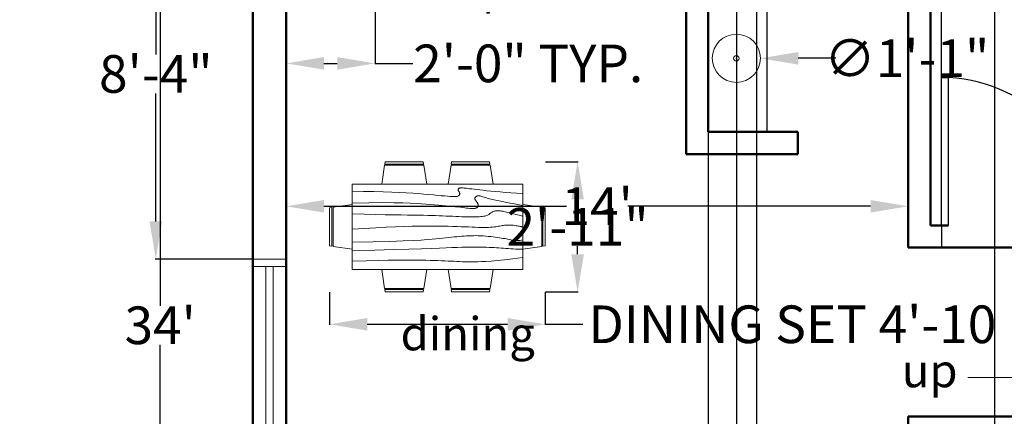
# Model space of a CAD drawing. Units: inches. Extents: x 20 to 3619, y 7 to 1288.
# Tile 2 of 4: x 3080 to 3346, y 967 to 1074. Entities that reach past the tile are written whole.
import ezdxf

# ---------------------------------------------------------------- set-up
doc = ezdxf.new("R2010")
doc.units = ezdxf.units.IN
doc.header["$MEASUREMENT"] = 0
for name, color, linetype, lineweight in [('A-ANNO-DIMS', 2, 'Continuous', 18), ('A-ANNO-SYMB', 7, 'Continuous', 18), ('A-ANNO-TEXT', 7, 'Continuous', 18), ('A-AREA-IDEN', 7, 'Continuous', 25), ('A-DOOR', 3, 'Continuous', 25), ('A-FLOR-CASE', 9, 'Continuous', 25), ('A-FLOR-FIXT', 9, 'Continuous', 18), ('A-FURN', 8, 'Continuous', 18), ('A-GLAZ', 4, 'Continuous', 18), ('A-WALL', 7, 'Continuous', 50)]:
    doc.layers.add(name, color=color, linetype=linetype, lineweight=lineweight)
doc.styles.get("Standard").update_dxf_attribs({"font": 'arial.ttf'})
doc.dimstyles.get("Standard").update_dxf_attribs({"dimtxt": 10.18, "dimasz": 10.18, "dimexe": 0.18, "dimexo": 0.0625, "dimgap": 0.09, "dimtad": 0, "dimtih": 1, "dimtoh": 1, "dimdec": 0, "dimzin": 0, "dimdsep": 46, "dimlunit": 3, "dimtxsty": 'Standard', "dimcen": 0.09, "dimadec": 0, "dimazin": 0, "dimtfac": 1, "dimtdec": 0, "dimtofl": 0, "dimtmove": 0, "dimatfit": 3, "dimfxl": 1, "dimtolj": 1, "dimtzin": 0, "dimarcsym": 0})

# ---------------------------------------------------------------- blocks, each defined once
blk = doc.blocks.new('*D4')
at = {"layer": 'A-ANNO-DIMS', "color": 0, "lineweight": -2, "transparency": 16777216}
for p, q in [((3142.66, 1195.69), (3117.53, 1195.69)), ((3117.71, 1185.51), (3117.71, 996.98)), ((3117.71, 797.87), (3117.71, 986.4)), ((3142.66, 787.69), (3117.53, 787.69))]:
    blk.add_line(p, q, dxfattribs=at)
at = {"layer": 'A-ANNO-DIMS', "color": 0, "transparency": 16777216}
for points in [[(3116.01, 1185.51), (3119.4, 1185.51), (3117.71, 1195.69)], [(3116.01, 797.87), (3119.4, 797.87), (3117.71, 787.69)]]:
    blk.add_solid(points, dxfattribs=at)
at = {"layer": 'Defpoints', "color": 0, "transparency": 16777216}
for p in [(3117.71, 1195.69), (3142.72, 1195.69), (3142.72, 787.69)]:
    blk.add_point(p, dxfattribs=at)
at = {"layer": 'A-ANNO-DIMS', "color": 0, "transparency": 16777216, "insert": (3117.71, 991.69), "char_height": 10.18, "attachment_point": 5}
blk.add_mtext("\\A1;34'", dxfattribs=at)
blk = doc.blocks.new('*U2')
for p, q in [((0, 0), (0, -6)), ((40, 0), (40, -6))]:
    blk.add_line(p, q)
blk.add_lwpolyline([(0, 0), (0, 40), (1.75, 40), (1.75, 0)], close=True)
blk.add_arc((0, 0), 40, 0, 90)
blk = doc.blocks.new('Dining Set - 36 x 72 in.')
for p, q in [((-22.2343, 26.00059), (-23.4847, 17.99762)), ((-22.2304, 26), (-5.7608, 26)), ((-22, 27.5), (-22.1562, 26.50042)), ((-5.8416, 26.5), (-22.1534, 26.5)), ((-22, 27.5), (-6, 27.5)), ((-5.8437, 26.49966), (-6, 27.5)), ((-4.5152, 17.99762), (-5.7655, 25.99926)), ((5.7657, 26.00059), (4.5153, 17.99762)), ((5.7696, 26), (22.2392, 26)), ((6, 27.5), (5.8438, 26.50042)), ((22.1584, 26.5), (5.8466, 26.5)), ((6, 27.5), (22, 27.5)), ((22.1563, 26.49966), (22, 27.5)), ((23.4848, 17.99762), (22.2345, 25.99926)), ((36, 18), (-36, 18)), ((-36, 18), (-36, -18)), ((36, -18), (36, 18)), ((-44.0006, 8.23428), (-35.9976, 9.48474)), ((44.0006, 8.23428), (35.9976, 9.48474)), ((-45.5, 8), (-44.5004, 8.15617)), ((-45.5, 8), (-45.5, -8)), ((-44.5, -8.15843), (-44.5, 8.15338)), ((-44, 8.23041), (-44, -8.23915)), ((44, 8.23041), (44, -8.23915)), ((44.5, -8.15843), (44.5, 8.15338)), ((45.5, 8), (44.5005, 8.15617)), ((45.5, 8), (45.5, -8)), ((-44.4997, -8.15631), (-45.5, -8)), ((-35.9976, -9.48476), (-43.9993, -8.2345)), ((35.9976, -9.48476), (43.9993, -8.2345)), ((44.4997, -8.15631), (45.5, -8)), ((-36, -18), (36, -18)), ((-22.2343, -26.0006), (-23.4847, -17.99762)), ((-4.5152, -17.99762), (-5.7655, -25.99928)), ((5.7657, -26.0006), (4.5153, -17.99762)), ((23.4848, -17.99762), (22.2345, -25.99928)), ((-22.2304, -26), (-5.7608, -26)), ((-22, -27.5), (-22.1562, -26.50044)), ((-5.8416, -26.5), (-22.1534, -26.5)), ((-22, -27.5), (-6, -27.5)), ((-5.8437, -26.49967), (-6, -27.5)), ((5.7696, -26), (22.2392, -26)), ((6, -27.5), (5.8438, -26.50044)), ((22.1584, -26.5), (5.8466, -26.5)), ((6, -27.5), (22, -27.5)), ((22.1563, -26.49967), (22, -27.5))]:
    blk.add_line(p, q)
for points in [[(-36, 15), (-31.1772, 14.97754), (-26.8079, 14.91406), (-22.8538, 14.81543), (-19.276, 14.6875), (-16.0362, 14.53613), (-13.0957, 14.36718), (-10.4159, 14.18652), (-7.9583, 14), (-5.6904, 13.81315), (-3.6035, 13.63021), (-1.6954, 13.45508), (0.0365, 13.29166), (1.5945, 13.14388), (2.9811, 13.01562), (4.1988, 12.9108), (5.25, 12.83333), (6.1393, 12.78613), (6.8802, 12.76823), (7.4883, 12.77767), (7.9792, 12.8125), (8.3685, 12.87077), (8.6719, 12.95052), (8.9049, 13.0498), (9.0833, 13.16666), (9.2205, 13.29899), (9.3216, 13.44401), (9.3895, 13.59879), (9.4271, 13.76041), (9.4373, 13.92594), (9.4232, 14.09245), (9.3875, 14.257), (9.3333, 14.41666), (9.2638, 14.56917), (9.1836, 14.71484), (9.0975, 14.85465), (9.0104, 14.98958), (8.9272, 15.1206), (8.8529, 15.2487), (8.7922, 15.37483), (8.75, 15.5), (8.7305, 15.62467), (8.7344, 15.74739), (8.7617, 15.86621), (8.8125, 15.97916), (8.8867, 16.08431), (8.9844, 16.17968), (9.1055, 16.26334), (9.25, 16.33333), (9.4189, 16.38802), (9.6172, 16.42708), (9.8506, 16.45052), (10.125, 16.45833), (10.4463, 16.45052), (10.8203, 16.42708), (11.2529, 16.38802), (11.75, 16.33333), (12.3184, 16.26318), (12.9694, 16.17838), (13.7151, 16.07991), (14.5677, 15.96875), (15.5395, 15.84586), (16.6426, 15.71224), (17.8893, 15.56884), (19.2917, 15.41666), (20.859, 15.25667), (22.5879, 15.08984), (24.4721, 14.91715), (26.5052, 14.73958), (28.6809, 14.5581), (30.9929, 14.3737), (33.4347, 14.18733), (36, 14)], [(-36, 10), (-28.9766, 10.14274), (-23.1725, 10.20442), (-18.4241, 10.19775), (-14.5677, 10.13541), (-11.4399, 10.03011), (-8.877, 9.89453), (-6.7154, 9.74137), (-4.7917, 9.58333), (-2.9698, 9.43082), (-1.2246, 9.28515), (0.4415, 9.14534), (2.026, 9.01041), (3.5266, 8.87939), (4.9408, 8.7513), (6.266, 8.62516), (7.5, 8.5), (8.6411, 8.37549), (9.6914, 8.2539), (10.6538, 8.13818), (11.5312, 8.03125), (12.3267, 7.93603), (13.043, 7.85547), (13.6831, 7.79248), (14.25, 7.75), (14.7471, 7.7303), (15.1797, 7.73307), (15.5537, 7.75732), (15.875, 7.80208), (16.1494, 7.86637), (16.3828, 7.94922), (16.5811, 8.04964), (16.75, 8.16666), (16.8944, 8.29915), (17.0143, 8.44531), (17.1089, 8.60319), (17.1771, 8.77083), (17.218, 8.94629), (17.2305, 9.1276), (17.2137, 9.31282), (17.1667, 9.5), (17.0895, 9.6875), (16.987, 9.875), (16.8649, 10.0625), (16.7292, 10.25), (16.5856, 10.4375), (16.4401, 10.625), (16.2985, 10.8125), (16.1667, 11), (16.05, 11.18733), (15.9518, 11.3737), (15.8752, 11.5581), (15.8229, 11.73958), (15.798, 11.91715), (15.8034, 12.08984), (15.842, 12.25667), (15.9167, 12.41666), (16.0295, 12.56836), (16.1784, 12.70833), (16.3605, 12.83268), (16.5729, 12.9375), (16.8127, 13.01888), (17.0768, 13.07291), (17.3625, 13.0957), (17.6667, 13.08333), (17.9894, 13.03312), (18.3418, 12.94726), (18.7382, 12.82918), (19.1927, 12.68229), (19.7195, 12.51001), (20.3327, 12.31575), (21.0465, 12.10294), (21.875, 11.875), (22.8357, 11.63354), (23.959, 11.37304), (25.2786, 11.08618), (26.8282, 10.76562), (28.6414, 10.40405), (30.752, 9.99414), (33.1936, 9.52856), (36, 9)], [(-36, 5.5), (-30.7157, 5.3348), (-26.069, 5.20963), (-21.9946, 5.11767), (-18.4271, 5.05208), (-15.3009, 5.00602), (-12.5508, 4.97265), (-10.1112, 4.94515), (-7.9167, 4.91666), (-5.909, 4.88167), (-4.0586, 4.83984), (-2.3429, 4.79215), (-0.7396, 4.73958), (0.7739, 4.6831), (2.22, 4.6237), (3.6213, 4.56233), (5, 4.5), (6.373, 4.43782), (7.7344, 4.3776), (9.0723, 4.32129), (10.375, 4.27083), (11.6309, 4.22819), (12.8281, 4.19531), (13.9551, 4.17415), (15, 4.16666), (15.954, 4.17448), (16.819, 4.19791), (17.6001, 4.23698), (18.3021, 4.29166), (18.9299, 4.36198), (19.4883, 4.44791), (19.9823, 4.54948), (20.4167, 4.66666), (20.7969, 4.79899), (21.1302, 4.94401), (21.4245, 5.09879), (21.6875, 5.26041), (21.9271, 5.42594), (22.1511, 5.59245), (22.3672, 5.757), (22.5834, 5.91666), (22.8065, 6.06868), (23.0404, 6.21093), (23.2879, 6.34147), (23.5521, 6.45833), (23.8358, 6.55957), (24.142, 6.64323), (24.4735, 6.70735), (24.8334, 6.75), (25.2235, 6.76969), (25.642, 6.76692), (26.0858, 6.74267), (26.5521, 6.69791), (27.0379, 6.63362), (27.5404, 6.55078), (28.0565, 6.45036), (28.5834, 6.33333), (29.1242, 6.19987), (29.7071, 6.04687), (30.3661, 5.87044), (31.1354, 5.66666), (32.0493, 5.43164), (33.142, 5.16146), (34.4475, 4.85221), (36, 4.5)], [(-36, -1), (-30.7915, -0.6591), (-26.0195, -0.38216), (-21.6519, -0.16284), (-17.6563, 0.00521), (-14.0005, 0.12833), (-10.6523, 0.21289), (-7.5796, 0.26522), (-4.75, 0.29166), (-2.134, 0.29793), (0.2878, 0.28711), (2.5317, 0.26163), (4.6146, 0.22396), (6.5529, 0.17651), (8.3633, 0.12174), (10.0623, 0.06209), (11.6667, 0), (13.1899, -0.06201), (14.6341, -0.1211), (15.9982, -0.17432), (17.2813, -0.21875), (18.4823, -0.25147), (19.6003, -0.26953), (20.6343, -0.27002), (21.5834, -0.25), (22.4481, -0.20768), (23.2357, -0.14584), (23.9549, -0.06836), (24.6146, 0.02083), (25.2235, 0.11784), (25.7904, 0.21875), (26.3241, 0.31966), (26.8334, 0.41666), (27.3265, 0.50618), (27.8099, 0.58593), (28.2894, 0.65397), (28.7709, 0.70833), (29.2601, 0.74707), (29.763, 0.76823), (30.2855, 0.76985), (30.8334, 0.75), (31.4088, 0.70784), (31.9994, 0.64713), (32.589, 0.57275), (33.1615, 0.48958), (33.7008, 0.4025), (34.1908, 0.3164), (34.6153, 0.23616), (34.9584, 0.16666), (35.2099, 0.11165), (35.3848, 0.07031), (35.504, 0.04069), (35.5886, 0.02083), (35.6594, 0.00879), (35.7377, 0.0026), (35.8442, 0.00032), (36, 0)], [(-36, -6.5), (-27.1843, -6.31267), (-20.084, -6.1263), (-14.469, -5.9419), (-10.1094, -5.76042), (-6.7752, -5.58285), (-4.2363, -5.41016), (-2.2629, -5.24333), (-0.625, -5.08334), (0.8708, -4.93099), (2.2715, -4.78646), (3.5872, -4.64974), (4.8281, -4.52084), (6.0046, -4.39974), (7.127, -4.28646), (8.2053, -4.18099), (9.25, -4.08334), (10.2705, -3.99382), (11.2734, -3.91407), (12.2647, -3.84603), (13.25, -3.79167), (14.2354, -3.75293), (15.2266, -3.73177), (16.2295, -3.73015), (17.25, -3.75), (18.2912, -3.79248), (19.3451, -3.85547), (20.4009, -3.93604), (21.4479, -4.03125), (22.4754, -4.13819), (23.4727, -4.25391), (24.4289, -4.37549), (25.3334, -4.5), (26.1785, -4.62492), (26.9694, -4.74935), (27.7145, -4.87281), (28.4219, -4.99479), (29.1, -5.11483), (29.7572, -5.23242), (30.4016, -5.34709), (31.0417, -5.45834), (31.6837, -5.56437), (32.3262, -5.65821), (32.9658, -5.73153), (33.599, -5.77604), (34.2224, -5.78345), (34.8327, -5.74545), (35.4264, -5.65373), (36, -5.5)], [(-36, -10), (-26.4022, -9.81299), (-18.4675, -9.62891), (-11.9839, -9.45069), (-6.7396, -9.28125), (-2.5226, -9.12354), (0.8789, -8.98047), (3.6769, -8.85498), (6.0833, -8.75), (8.2767, -8.66765), (10.3021, -8.60677), (12.1712, -8.56543), (13.8958, -8.54167), (15.4876, -8.53353), (16.9583, -8.53907), (18.3197, -8.55632), (19.5834, -8.58334), (20.7616, -8.61841), (21.8685, -8.66081), (22.9188, -8.71004), (23.9271, -8.76563), (24.9081, -8.82707), (25.8763, -8.89388), (26.8465, -8.96558), (27.8334, -9.04167), (28.8474, -9.12118), (29.8828, -9.20117), (30.93, -9.27824), (31.9792, -9.34896), (33.0205, -9.40991), (34.0443, -9.45768), (35.0407, -9.48885), (36, -9.5)], [(-36, -14.5), (-30.0881, -14.33513), (-25.0332, -14.21224), (-20.7312, -14.12647), (-17.0781, -14.07292), (-13.97, -14.04671), (-11.3027, -14.04297), (-8.9724, -14.05681), (-6.875, -14.08334), (-4.9224, -14.11833), (-3.0905, -14.16016), (-1.3709, -14.20785), (0.2448, -14.26042), (1.7647, -14.3169), (3.1973, -14.3763), (4.5507, -14.43767), (5.8333, -14.5), (7.0554, -14.5621), (8.235, -14.62175), (9.3922, -14.67652), (10.5469, -14.72396), (11.7192, -14.76164), (12.929, -14.78711), (14.1965, -14.79794), (15.5417, -14.79167), (16.9933, -14.76424), (18.6152, -14.70508), (20.4804, -14.60197), (22.6615, -14.44271), (25.2312, -14.21509), (28.2624, -13.9069), (31.8277, -13.50594), (36, -13)]]:
    blk.add_lwpolyline(points)
blk = doc.blocks.new('*D10')
at = {"layer": 'A-ANNO-DIMS', "color": 0, "lineweight": -2, "transparency": 16777216}
for p, q in [((3151.72, 1044.4), (3151.72, 1023.68)), ((3319.72, 1044.4), (3319.72, 1023.68)), ((3161.9, 1023.86), (3227.47, 1023.86)), ((3309.54, 1023.86), (3243.97, 1023.86))]:
    blk.add_line(p, q, dxfattribs=at)
at = {"layer": 'A-ANNO-DIMS', "color": 0, "transparency": 16777216}
for points in [[(3161.9, 1025.55), (3161.9, 1022.16), (3151.72, 1023.86)], [(3309.54, 1025.55), (3309.54, 1022.16), (3319.72, 1023.86)]]:
    blk.add_solid(points, dxfattribs=at)
at = {"layer": 'Defpoints', "color": 0, "transparency": 16777216}
for p in [(3151.72, 1044.47), (3319.72, 1044.47), (3319.72, 1023.86)]:
    blk.add_point(p, dxfattribs=at)
at = {"layer": 'A-ANNO-DIMS', "color": 0, "transparency": 16777216, "insert": (3235.72, 1023.86), "char_height": 10.18, "attachment_point": 5}
blk.add_mtext("\\A1;14'", dxfattribs=at)
blk = doc.blocks.new('WIN-48IN-PLAN')
for p, q in [((0, 0), (0, 9)), ((2, 0), (2, 9)), ((50, 0), (50, 9)), ((52, 0), (52, 9)), ((2, 5.5), (50, 5.5)), ((2, 3.5), (50, 3.5))]:
    blk.add_line(p, q)
blk = doc.blocks.new('*D25')
at = {"layer": 'A-ANNO-DIMS', "color": 0, "lineweight": -2, "transparency": 16777216}
for p, q in [((3151.72, 1078.63), (3151.72, 1062.31)), ((3175.72, 1078.63), (3175.72, 1062.31)), ((3161.9, 1062.49), (3165.54, 1062.49)), ((3175.72, 1062.49), (3185.9, 1062.49))]:
    blk.add_line(p, q, dxfattribs=at)
at = {"layer": 'A-ANNO-DIMS', "color": 0, "transparency": 16777216}
for points in [[(3161.9, 1064.19), (3161.9, 1060.8), (3151.72, 1062.49)], [(3165.54, 1064.19), (3165.54, 1060.8), (3175.72, 1062.49)]]:
    blk.add_solid(points, dxfattribs=at)
at = {"layer": 'Defpoints', "color": 0, "transparency": 16777216}
for p in [(3151.72, 1078.69), (3175.72, 1078.69), (3175.72, 1062.49)]:
    blk.add_point(p, dxfattribs=at)
at = {"layer": 'A-ANNO-DIMS', "color": 0, "transparency": 16777216, "insert": (3217.1, 1062.49), "char_height": 10.18, "attachment_point": 5}
blk.add_mtext('\\A1;2\'-0" TYP.', dxfattribs=at)
blk = doc.blocks.new('*D28')
at = {"layer": 'A-ANNO-DIMS', "color": 0, "lineweight": -2, "transparency": 16777216}
for p, q in [((3163.42, 1000.64), (3163.42, 991.78)), ((3221.69, 1000.64), (3221.69, 991.78)), ((3173.6, 991.96), (3211.51, 991.96)), ((3221.69, 991.96), (3231.87, 991.96))]:
    blk.add_line(p, q, dxfattribs=at)
at = {"layer": 'A-ANNO-DIMS', "color": 0, "transparency": 16777216}
for points in [[(3173.6, 993.66), (3173.6, 990.26), (3163.42, 991.96)], [(3211.51, 993.66), (3211.51, 990.26), (3221.69, 991.96)]]:
    blk.add_solid(points, dxfattribs=at)
at = {"layer": 'Defpoints', "color": 0, "transparency": 16777216}
for p in [(3163.42, 1000.7), (3221.69, 1000.7), (3221.69, 991.96)]:
    blk.add_point(p, dxfattribs=at)
at = {"layer": 'A-ANNO-DIMS', "color": 0, "transparency": 16777216, "insert": (3303.72, 991.96), "char_height": 10.18, "attachment_point": 5}
blk.add_mtext('\\A1;DINING SET 4\'-10 1/2"', dxfattribs=at)
blk = doc.blocks.new('*D29')
at = {"layer": 'A-ANNO-DIMS', "color": 0, "lineweight": -2, "transparency": 16777216}
for p, q in [((3221.76, 1035.92), (3230.61, 1035.92)), ((3230.43, 1025.74), (3230.43, 1023.51)), ((3230.43, 1010.88), (3230.43, 1013.11)), ((3221.76, 1000.7), (3230.61, 1000.7))]:
    blk.add_line(p, q, dxfattribs=at)
at = {"layer": 'A-ANNO-DIMS', "color": 0, "transparency": 16777216}
for points in [[(3228.74, 1025.74), (3232.13, 1025.74), (3230.43, 1035.92)], [(3228.74, 1010.88), (3232.13, 1010.88), (3230.43, 1000.7)]]:
    blk.add_solid(points, dxfattribs=at)
at = {"layer": 'Defpoints', "color": 0, "transparency": 16777216}
for p in [(3221.69, 1035.92), (3230.43, 1035.92), (3221.69, 1000.7)]:
    blk.add_point(p, dxfattribs=at)
at = {"layer": 'A-ANNO-DIMS', "color": 0, "transparency": 16777216, "insert": (3230.43, 1018.31), "char_height": 10.18, "attachment_point": 5}
blk.add_mtext('\\A1;2\'-11"', dxfattribs=at)
blk = doc.blocks.new('*D30')
at = {"layer": 'A-ANNO-DIMS', "color": 0, "lineweight": -2, "transparency": 16777216}
for p, q in [((3240.92, 1120.08), (3236.84, 1120.08)), ((3237.02, 1109.9), (3237.02, 1103.86)), ((3240.92, 1093.68), (3236.84, 1093.68)), ((3237.02, 1093.68), (3237.02, 1083.5)), ((3237.02, 1083.5), (3226.84, 1083.5))]:
    blk.add_line(p, q, dxfattribs=at)
at = {"layer": 'A-ANNO-DIMS', "color": 0, "transparency": 16777216}
for points in [[(3235.33, 1109.9), (3238.72, 1109.9), (3237.02, 1120.08)], [(3235.33, 1103.86), (3238.72, 1103.86), (3237.02, 1093.68)]]:
    blk.add_solid(points, dxfattribs=at)
at = {"layer": 'Defpoints', "color": 0, "transparency": 16777216}
for p in [(3240.98, 1120.08), (3237.02, 1093.68), (3240.98, 1093.68)]:
    blk.add_point(p, dxfattribs=at)
at = {"layer": 'A-ANNO-DIMS', "color": 0, "transparency": 16777216, "insert": (3151.83, 1083.5), "char_height": 10.18, "attachment_point": 5}
blk.add_mtext('\\A1;DOUBLE SINK 2\'-2 1/2"', dxfattribs=at)
blk = doc.blocks.new('*D40')
at = {"layer": 'A-ANNO-DIMS', "color": 0, "lineweight": -2, "transparency": 16777216}
for p, q in [((3332.89, 1272.89), (3322.71, 1272.89)), ((3343.07, 796.76), (3343.07, 1273.07)), ((3382.22, 796.76), (3382.22, 1273.07)), ((3392.4, 1272.89), (3402.58, 1272.89))]:
    blk.add_line(p, q, dxfattribs=at)
at = {"layer": 'A-ANNO-DIMS', "color": 0, "transparency": 16777216}
for points in [[(3332.89, 1274.59), (3332.89, 1271.2), (3343.07, 1272.89)], [(3392.4, 1274.59), (3392.4, 1271.2), (3382.22, 1272.89)]]:
    blk.add_solid(points, dxfattribs=at)
at = {"layer": 'Defpoints', "color": 0, "transparency": 16777216}
for p in [(3382.22, 1272.89), (3343.07, 796.69), (3382.22, 796.69)]:
    blk.add_point(p, dxfattribs=at)
at = {"layer": 'A-ANNO-DIMS', "color": 0, "transparency": 16777216, "insert": (3362.64, 1272.89), "char_height": 10.18, "attachment_point": 5}
blk.add_mtext('\\A1;3\'-3"', dxfattribs=at)
blk = doc.blocks.new('*D41')
at = {"layer": 'A-ANNO-DIMS', "color": 0, "lineweight": -2, "transparency": 16777216}
for p, q in [((3263.21, 1272.89), (3253.03, 1272.89)), ((3273.39, 796.76), (3273.39, 1273.07)), ((3343.07, 796.76), (3343.07, 1273.07)), ((3353.25, 1272.89), (3363.43, 1272.89))]:
    blk.add_line(p, q, dxfattribs=at)
at = {"layer": 'A-ANNO-DIMS', "color": 0, "transparency": 16777216}
for points in [[(3263.21, 1274.59), (3263.21, 1271.2), (3273.39, 1272.89)], [(3353.25, 1274.59), (3353.25, 1271.2), (3343.07, 1272.89)]]:
    blk.add_solid(points, dxfattribs=at)
at = {"layer": 'Defpoints', "color": 0, "transparency": 16777216}
for p in [(3343.07, 1272.89), (3273.39, 796.69), (3343.07, 796.69)]:
    blk.add_point(p, dxfattribs=at)
at = {"layer": 'A-ANNO-DIMS', "color": 0, "transparency": 16777216, "insert": (3308.23, 1272.89), "char_height": 10.18, "attachment_point": 5}
blk.add_mtext('\\A1;5\'-9 1/2"', dxfattribs=at)
blk = doc.blocks.new('*D43')
at = {"layer": 'A-ANNO-DIMS', "color": 0, "lineweight": -2, "transparency": 16777216}
for p, q in [((3142.66, 1109.69), (3116.34, 1109.69)), ((3116.52, 1099.51), (3116.52, 1064.93)), ((3116.52, 1019.77), (3116.52, 1054.35)), ((3142.66, 1009.59), (3116.34, 1009.59))]:
    blk.add_line(p, q, dxfattribs=at)
at = {"layer": 'A-ANNO-DIMS', "color": 0, "transparency": 16777216}
for points in [[(3114.82, 1099.51), (3118.21, 1099.51), (3116.52, 1109.69)], [(3114.82, 1019.77), (3118.21, 1019.77), (3116.52, 1009.59)]]:
    blk.add_solid(points, dxfattribs=at)
at = {"layer": 'Defpoints', "color": 0, "transparency": 16777216}
for p in [(3116.52, 1109.69), (3142.72, 1109.69), (3142.72, 1009.59)]:
    blk.add_point(p, dxfattribs=at)
at = {"layer": 'A-ANNO-DIMS', "color": 0, "transparency": 16777216, "insert": (3116.52, 1059.64), "char_height": 10.18, "attachment_point": 5}
blk.add_mtext('\\A1;8\'-4"', dxfattribs=at)
blk = doc.blocks.new('*D47')
at = {"layer": 'A-ANNO-DIMS', "color": 0, "lineweight": -2, "transparency": 16777216}
for p, q in [((3265.72, 1186.63), (3265.72, 701.31)), ((3278.72, 1186.63), (3278.72, 701.31)), ((3255.54, 701.49), (3245.36, 701.49)), ((3288.9, 701.49), (3299.08, 701.49))]:
    blk.add_line(p, q, dxfattribs=at)
at = {"layer": 'A-ANNO-DIMS', "color": 0, "transparency": 16777216}
for points in [[(3255.54, 703.19), (3255.54, 699.8), (3265.72, 701.49)], [(3288.9, 703.19), (3288.9, 699.8), (3278.72, 701.49)]]:
    blk.add_solid(points, dxfattribs=at)
at = {"layer": 'Defpoints', "color": 0, "transparency": 16777216}
for p in [(3265.72, 1186.69), (3278.72, 1186.69), (3278.72, 701.49)]:
    blk.add_point(p, dxfattribs=at)
at = {"layer": 'A-ANNO-DIMS', "color": 0, "transparency": 16777216, "insert": (3312.22, 701.49), "char_height": 10.18, "attachment_point": 5}
blk.add_mtext('\\A1;1\'-1"', dxfattribs=at)
blk = doc.blocks.new('*D52')
at = {"layer": 'A-ANNO-DIMS', "color": 0, "lineweight": -2, "transparency": 16777216}
for p, q in [((3318.54, 1272.89), (3308.36, 1272.89)), ((3328.72, 1018.76), (3328.72, 1273.07)), ((3368.72, 1018.76), (3368.72, 1273.07)), ((3378.9, 1272.89), (3389.08, 1272.89))]:
    blk.add_line(p, q, dxfattribs=at)
at = {"layer": 'A-ANNO-DIMS', "color": 0, "transparency": 16777216}
for points in [[(3318.54, 1274.59), (3318.54, 1271.2), (3328.72, 1272.89)], [(3378.9, 1274.59), (3378.9, 1271.2), (3368.72, 1272.89)]]:
    blk.add_solid(points, dxfattribs=at)
at = {"layer": 'Defpoints', "color": 0, "transparency": 16777216}
for p in [(3368.72, 1272.89), (3328.72, 1018.69), (3368.72, 1018.69)]:
    blk.add_point(p, dxfattribs=at)
at = {"layer": 'A-ANNO-DIMS', "color": 0, "transparency": 16777216, "insert": (3348.72, 1272.89), "char_height": 10.18, "attachment_point": 5}
blk.add_mtext('\\A1;3\'-4"', dxfattribs=at)
blk = doc.blocks.new('*D53')
at = {"layer": 'A-ANNO-DIMS', "color": 0, "lineweight": -2, "transparency": 16777216}
for p, q in [((3273.22, 1063.87), (3273.4, 1063.87)), ((3273.31, 1063.78), (3273.31, 1063.96)), ((3300.18, 1063.87), (3290, 1063.87))]:
    blk.add_line(p, q, dxfattribs=at)
at = {"layer": 'A-ANNO-DIMS', "color": 0, "transparency": 16777216}
blk.add_solid([(3290, 1065.56), (3290, 1062.17), (3279.82, 1063.87)], dxfattribs=at)
at = {"layer": 'Defpoints', "color": 0, "transparency": 16777216}
for p in [(3266.8, 1063.87), (3279.82, 1063.87)]:
    blk.add_point(p, dxfattribs=at)
at = {"layer": 'A-ANNO-DIMS', "color": 0, "transparency": 16777216, "insert": (3319.34, 1063.87), "char_height": 10.18, "attachment_point": 5}
blk.add_mtext('\\A1;∅1\'-1"', dxfattribs=at)

msp = doc.modelspace()

# ---------------------------------------------------------------- linework, layer by layer
at = {"layer": 'A-ANNO-SYMB'}
msp.add_line((3335.85, 977.55), (3352.72, 977.55), dxfattribs=at)
at = {"layer": 'A-FLOR-CASE'}
msp.add_line((3281.56, 1084.69), (3281.56, 1043.99), dxfattribs=at)
at = {"layer": 'A-FLOR-FIXT'}
for radius in [6.51, 0.74]:
    msp.add_circle((3273.31, 1063.87), radius, dxfattribs=at)
at = {"layer": 'A-GLAZ'}
msp.add_line((3148.22, 1007.59), (3148.22, 959.59), dxfattribs=at)
at = {"layer": 'A-WALL'}
for p, q in [((3142.72, 787.69), (3142.72, 1195.69)), ((3319.72, 1012.69), (3319.72, 1186.69)), ((3319.72, 1012.69), (3319.72, 1186.69)), ((3325.72, 1018.69), (3325.72, 1186.69)), ((3151.72, 796.69), (3151.72, 1078.69)), ((3259.72, 1078.69), (3259.72, 1037.99)), ((3265.72, 1078.69), (3265.72, 1043.99)), ((3265.72, 1043.99), (3289.89, 1043.99)), ((3289.89, 1043.99), (3289.89, 1037.99)), ((3259.72, 1037.99), (3289.89, 1037.99)), ((3325.72, 1018.69), (3330.47, 1018.69)), ((3319.72, 1012.69), (3328.72, 1012.69)), ((3328.72, 1012.69), (3445.72, 1012.69)), ((3319.72, 958.08), (3319.72, 967.08)), ((3445.72, 967.08), (3319.72, 967.08))]:
    msp.add_line(p, q, dxfattribs=at)

# ---------------------------------------------------------------- block references
at = {"layer": 'A-DOOR'}
msp.add_blockref('*U2', (3328.72, 1018.69), dxfattribs=at)
at = {"layer": 'A-FURN', "xscale": 0.6403747421773762, "yscale": 0.6403747421773762, "zscale": 0.6403747421773762}
msp.add_blockref('Dining Set - 36 x 72 in.', (3192.56, 1018.31), dxfattribs=at)
at = {"layer": 'A-GLAZ', "rotation": 89.99999999999845}
msp.add_blockref('WIN-48IN-PLAN', (3151.72, 957.59), dxfattribs=at)

# ---------------------------------------------------------------- texts
at = {"layer": 'A-ANNO-TEXT', "insert": (3317.99, 983.94), "char_height": 9, "attachment_point": 1}
msp.add_mtext_dynamic_manual_height_columns('up ', width=17.3739, gutter_width=1, heights=[0], dxfattribs=at)
at = {"layer": 'A-AREA-IDEN', "insert": (3182.62, 993.93), "char_height": 9, "attachment_point": 1}
msp.add_mtext_dynamic_manual_height_columns('dining ', width=17.3739, gutter_width=1, heights=[0], dxfattribs=at)

# ---------------------------------------------------------------- dimensions: what is measured, and where the dimension line sits
at = {"layer": 'A-ANNO-DIMS'}
for base, p1, p2, override, picture, middle in [((3343.07, 1272.89), (3273.39, 796.69), (3343.07, 796.69), {"dimdec": 1, "dimlfac": 1, "dimrnd": 0, "dimzin": 1, "dimdsep": 46, "dimlunit": 4, "dimfrac": 2}, '*D41', (3308.23, 1272.89)), ((3368.72, 1272.89), (3328.72, 1018.69), (3368.72, 1018.69), {"dimdec": 1, "dimlfac": 1, "dimrnd": 0, "dimzin": 1, "dimdsep": 46, "dimlunit": 4, "dimfrac": 2}, '*D52', (3348.72, 1272.89)), ((3382.2188, 1272.8933), (3343.0711, 796.6933), (3382.2188, 796.6933), {"dimdec": 1, "dimlfac": 1, "dimrnd": 0, "dimzin": 1, "dimdsep": 46, "dimlunit": 4, "dimfrac": 2}, '*D40', (3362.6449, 1272.8933)), ((3278.72, 701.49), (3265.72, 1186.69), (3278.72, 1186.69), {"dimdec": 1, "dimlfac": 1, "dimrnd": 0, "dimzin": 1, "dimdsep": 46, "dimlunit": 4, "dimfrac": 2}, '*D47', (3312.22, 701.49)), ((3319.72, 1023.86), (3151.72, 1044.47), (3319.72, 1044.47), {"dimclrd": 0, "dimclre": 0, "dimclrt": 0}, '*D10', (3235.72, 1023.86))]:
    dim = msp.add_linear_dim(base=base, p1=p1, p2=p2, dimstyle='Standard', override=override, dxfattribs=at)
    dim.commit()
    dim.dimension.update_dxf_attribs({"geometry": picture, "text_midpoint": middle})
for base, p1, p2, override, picture, middle in [((3117.71, 1195.69), (3142.72, 787.69), (3142.72, 1195.69), {"dimclrd": 0, "dimclre": 0, "dimclrt": 0}, '*D4', (3117.71, 991.69)), ((3116.52, 1109.69), (3142.72, 1009.59), (3142.72, 1109.69), {"dimdec": 1, "dimlfac": 1, "dimrnd": 0, "dimzin": 1, "dimdsep": 46, "dimlunit": 4, "dimfrac": 2}, '*D43', (3116.52, 1059.64)), ((3230.43, 1035.92), (3221.69, 1000.7), (3221.69, 1035.92), {"dimdec": 1, "dimlfac": 1, "dimrnd": 0, "dimzin": 1, "dimdsep": 46, "dimlunit": 4, "dimfrac": 2}, '*D29', (3230.43, 1018.31))]:
    dim = msp.add_linear_dim(base=base, p1=p1, p2=p2, angle=90, dimstyle='Standard', override=override, dxfattribs=at)
    dim.commit()
    dim.dimension.update_dxf_attribs({"geometry": picture, "text_midpoint": middle})
dim = msp.add_linear_dim(base=(3237.02, 1093.68), p1=(3240.98, 1120.08), p2=(3240.98, 1093.68), angle=270, text='DOUBLE SINK <>', dimstyle='Standard', override={"dimdec": 1, "dimlfac": 1, "dimrnd": 0, "dimzin": 1, "dimdsep": 46, "dimlunit": 4, "dimfrac": 2}, dxfattribs=at)
dim.commit()
dim.dimension.update_dxf_attribs({"geometry": '*D30', "text_midpoint": (3151.83, 1083.5)})
for base, p1, p2, text, picture, middle in [((3175.72, 1062.49), (3151.72, 1078.69), (3175.72, 1078.69), '<> TYP.', '*D25', (3217.1, 1062.49)), ((3221.69, 991.96), (3163.42, 1000.7), (3221.69, 1000.7), 'DINING SET <>', '*D28', (3303.72, 991.96))]:
    dim = msp.add_linear_dim(base=base, p1=p1, p2=p2, text=text, dimstyle='Standard', override={"dimdec": 1, "dimlfac": 1, "dimrnd": 0, "dimzin": 1, "dimdsep": 46, "dimlunit": 4, "dimfrac": 2}, dxfattribs=at)
    dim.commit()
    dim.dimension.update_dxf_attribs({"geometry": picture, "text_midpoint": middle})
dim = msp.add_diameter_dim_2p(p1=(3266.8, 1063.87), p2=(3279.82, 1063.87), dimstyle='Standard', override={"dimdec": 1, "dimlfac": 1, "dimrnd": 0, "dimzin": 1, "dimdsep": 46, "dimlunit": 4, "dimfrac": 2}, dxfattribs=at)
dim.commit()
dim.dimension.update_dxf_attribs({"geometry": '*D53', "text_midpoint": (3300.18, 1063.87), "dimtype": 163})

doc.saveas('drawing.dxf')
